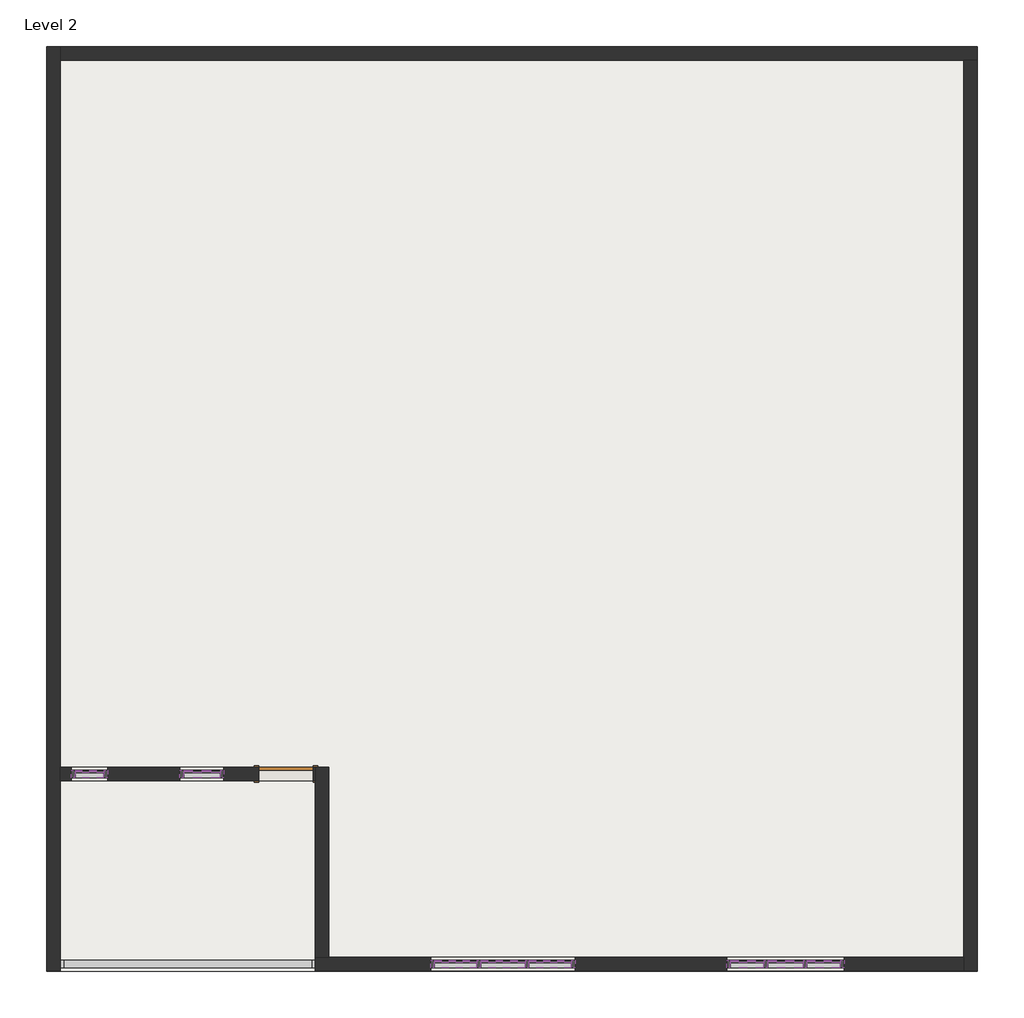
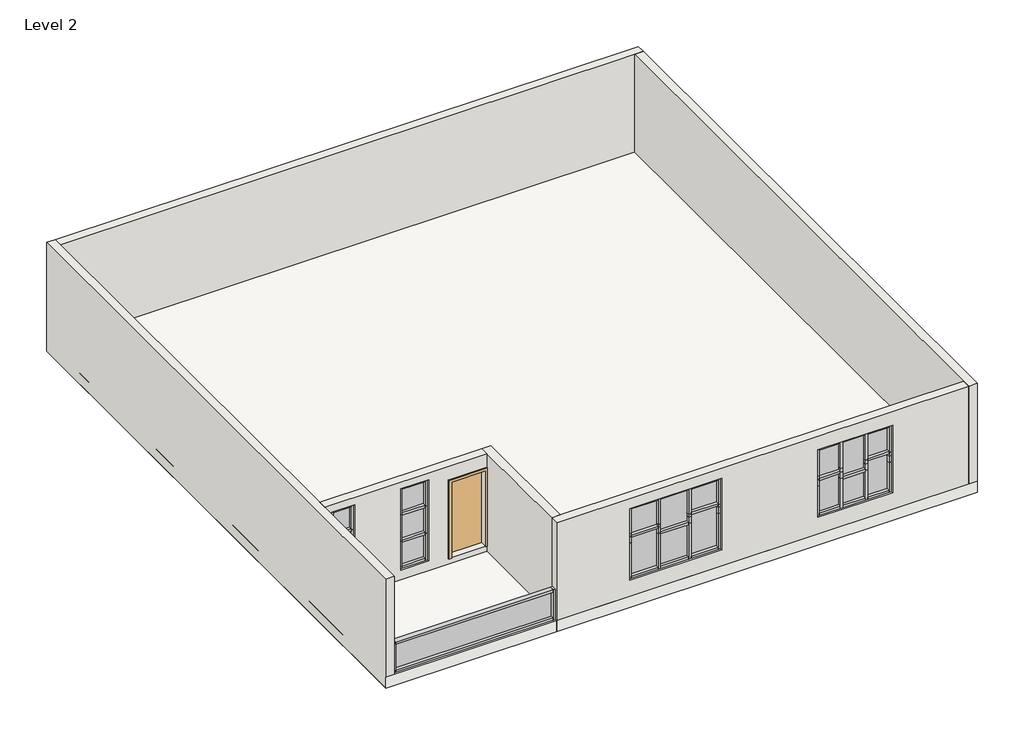
# One storey: 74 members, 19 plates, 6 walls, 1 door, 1 roof.
"""IFC4 building model written with IfcOpenShell, lengths in millimetres."""

from ifc_helpers import new_model, si_unit, frame, origin, place, context, project, spatial, polyline, outline, extrude, faceted_brep, transform, mapped, element, save
from components import door_0ca8825f, member_3d7cb871, member_6103f85b, member_00d00b53, member_86293703, member_cfc5edb3, member_a400357f, member_6f432376, member_abeaf8ac, member_798d6cad, member_9d02be77, member_7007ad49, member_86d06fe4, member_323df77c, member_fb13da3b, member_d92184fb, member_86adc6a2, member_2118ea0c, member_92f44db0, member_44fc35f8, member_a1032ffb, member_2251cb41, member_9a1a11af, member_7982986b, member_74f949a7, member_09784a4a, member_ee585a1e, member_f8dc38bf, member_3f0e0172, member_39ae6cfa, member_86c371d5, system_panel_glazed_a2969b70, system_panel_glazed_06a12247, system_panel_glazed_4710a741, system_panel_glazed_6f1997f1, system_panel_glazed_71cd45ac, system_panel_glazed_e7b2ff25, system_panel_glazed_4fbea3b4, system_panel_glazed_12683933, system_panel_glazed_3f655f72, system_panel_glazed_72d2109d, system_panel_glazed_9ec27a3c, system_panel_glazed_53cab8c3, system_panel_glazed_a0fb9759, system_panel_glazed_76104635, system_panel_glazed_cd499e62, system_panel_glazed_4a2f6317, system_panel_glazed_4f9242a6

model = new_model("IFC4")

# Units and contexts
model_context = context("Model", 3, world=origin())
ifc_project = project(units=[si_unit("LENGTHUNIT", "METRE", prefix="MILLI")], contexts=[model_context])

# Site, building, storey
site = spatial("IfcSite", under=ifc_project)
building = spatial("IfcBuilding", under=site)
storey = spatial("IfcBuildingStorey", under=building, Name="Level 2", Elevation=3048.0)

# Door
placement = place(None, origin())
door_shape = door_0ca8825f(model_context)
element("IfcDoor", 1, ObjectType="Single-Flush : 36\" x 84\"", at=placement, inside=storey, context=model_context, shape_type="MappedRepresentation", body=[
    mapped(door_shape, transform((-15283.714323, -10539.4538163, 3505.2), x_axis=(1.0, 0.0, 0.0), y_axis=(0.0, 1.0, 0.0), z_axis=(0.0, 0.0, 1.0))),
])

# Members
member_shape = member_3d7cb871(model_context)
element("IfcMember", 2, ObjectType="Rectangular Mullion : 2.5\" x 5\" rectangular", at=placement, inside=storey, context=model_context, shape_type="MappedRepresentation", body=[
    mapped(member_shape, transform((-12845.314323, -13739.8538163, 5060.9680142), x_axis=(-1.0, 0.0, 0.0), y_axis=(0.0, -1.0, 0.0), z_axis=(0.0, 0.0, 1.0))),
])
member_2_shape = member_6103f85b(model_context)
element("IfcMember", 3, ObjectType="Rectangular Mullion : 2.5\" x 5\" rectangular", at=placement, inside=storey, context=model_context, shape_type="MappedRepresentation", body=[
    mapped(member_2_shape, transform((-7225.564323, -13739.8538163, 4831.3724927), x_axis=(0.0, 0.0, 1.0), y_axis=(0.0, -1.0, 0.0), z_axis=(1.0, 0.0, 0.0))),
])
element("IfcMember", 4, ObjectType="Rectangular Mullion : 2.5\" x 5\" rectangular", at=placement, inside=storey, context=model_context, shape_type="MappedRepresentation", body=[
    mapped(member_2_shape, transform((-5936.514323, -13739.8538163, 4932.9724927), x_axis=(0.0, 0.0, 1.0), y_axis=(0.0, -1.0, 0.0), z_axis=(1.0, 0.0, 0.0))),
])
member_3_shape = member_00d00b53(model_context)
element("IfcMember", 5, ObjectType="Rectangular Mullion : 2.5\" x 5\" rectangular", at=placement, inside=storey, context=model_context, shape_type="MappedRepresentation", body=[
    mapped(member_3_shape, transform((-12032.514323, -13739.8538163, 4984.7680142), x_axis=(1.0, 0.0, 0.0), y_axis=(0.0, -1.0, 0.0), z_axis=(0.0, 0.0, -1.0))),
])
member_4_shape = member_86293703(model_context)
element("IfcMember", 6, ObjectType="Rectangular Mullion : 2.5\" x 5\" rectangular", at=placement, inside=storey, context=model_context, shape_type="MappedRepresentation", body=[
    mapped(member_4_shape, transform((-6565.164323, -13739.8538163, 4653.5724927), x_axis=(0.0, 0.0, 1.0), y_axis=(0.0, -1.0, 0.0), z_axis=(1.0, 0.0, 0.0))),
])
member_5_shape = member_cfc5edb3(model_context)
element("IfcMember", 7, ObjectType="Rectangular Mullion : 2.5\" x 5\" rectangular", at=placement, inside=storey, context=model_context, shape_type="MappedRepresentation", body=[
    mapped(member_5_shape, transform((-7193.814323, -13739.8538163, 4831.3724927), x_axis=(1.0, 0.0, 0.0), y_axis=(0.0, -1.0, 0.0), z_axis=(0.0, 0.0, -1.0))),
])
element("IfcMember", 8, ObjectType="Rectangular Mullion : 2.5\" x 5\" rectangular", at=placement, inside=storey, context=model_context, shape_type="MappedRepresentation", body=[
    mapped(member_3_shape, transform((-11219.714323, -13739.8538163, 4984.7680142), x_axis=(1.0, 0.0, 0.0), y_axis=(0.0, -1.0, 0.0), z_axis=(0.0, 0.0, -1.0))),
])
member_6_shape = member_a400357f(model_context)
element("IfcMember", 9, ObjectType="Rectangular Mullion : 2.5\" x 5\" rectangular", at=placement, inside=storey, context=model_context, shape_type="MappedRepresentation", body=[
    mapped(member_6_shape, transform((-7162.064323, -13739.8538163, 3815.3724927), x_axis=(0.0, 0.0, -1.0), y_axis=(0.0, -1.0, 0.0), z_axis=(-1.0, 0.0, 0.0))),
])
member_7_shape = member_6f432376(model_context)
element("IfcMember", 10, ObjectType="Rectangular Mullion : 2.5\" x 5\" rectangular", at=placement, inside=storey, context=model_context, shape_type="MappedRepresentation", body=[
    mapped(member_7_shape, transform((-6501.664323, -13739.8538163, 3815.3724927), x_axis=(0.0, 0.0, -1.0), y_axis=(0.0, -1.0, 0.0), z_axis=(-1.0, 0.0, 0.0))),
])
element("IfcMember", 11, ObjectType="Rectangular Mullion : 2.5\" x 5\" rectangular", at=placement, inside=storey, context=model_context, shape_type="MappedRepresentation", body=[
    mapped(member_7_shape, transform((-7790.714323, -13739.8538163, 3815.3724927), x_axis=(0.0, 0.0, -1.0), y_axis=(0.0, -1.0, 0.0), z_axis=(-1.0, 0.0, 0.0))),
])
element("IfcMember", 12, ObjectType="Rectangular Mullion : 2.5\" x 5\" rectangular", at=placement, inside=storey, context=model_context, shape_type="MappedRepresentation", body=[
    mapped(member_7_shape, transform((-7225.564323, -13739.8538163, 5713.2534541), x_axis=(0.0, 0.0, 1.0), y_axis=(0.0, -1.0, 0.0), z_axis=(1.0, 0.0, 0.0))),
])
element("IfcMember", 13, ObjectType="Rectangular Mullion : 2.5\" x 5\" rectangular", at=placement, inside=storey, context=model_context, shape_type="MappedRepresentation", body=[
    mapped(member_7_shape, transform((-5936.514323, -13739.8538163, 5713.2534541), x_axis=(0.0, 0.0, 1.0), y_axis=(0.0, -1.0, 0.0), z_axis=(1.0, 0.0, 0.0))),
])
element("IfcMember", 14, ObjectType="Rectangular Mullion : 2.5\" x 5\" rectangular", at=placement, inside=storey, context=model_context, shape_type="MappedRepresentation", body=[
    mapped(member_6_shape, transform((-6565.164323, -13739.8538163, 5713.2534541), x_axis=(0.0, 0.0, 1.0), y_axis=(0.0, -1.0, 0.0), z_axis=(1.0, 0.0, 0.0))),
])
member_8_shape = member_abeaf8ac(model_context)
element("IfcMember", 15, ObjectType="Rectangular Mullion : 2.5\" x 5\" rectangular", at=placement, inside=storey, context=model_context, shape_type="MappedRepresentation", body=[
    mapped(member_8_shape, transform((-12064.264323, -13739.8538163, 4984.7680142), x_axis=(0.0, 0.0, 1.0), y_axis=(0.0, -1.0, 0.0), z_axis=(1.0, 0.0, 0.0))),
])
element("IfcMember", 16, ObjectType="Rectangular Mullion : 2.5\" x 5\" rectangular", at=placement, inside=storey, context=model_context, shape_type="MappedRepresentation", body=[
    mapped(member_8_shape, transform((-10470.414323, -13739.8538163, 5060.9680142), x_axis=(0.0, 0.0, 1.0), y_axis=(0.0, -1.0, 0.0), z_axis=(1.0, 0.0, 0.0))),
])
member_9_shape = member_798d6cad(model_context)
element("IfcMember", 17, ObjectType="Rectangular Mullion : 2.5\" x 5\" rectangular", at=placement, inside=storey, context=model_context, shape_type="MappedRepresentation", body=[
    mapped(member_9_shape, transform((-11251.464323, -13739.8538163, 4806.9680142), x_axis=(0.0, 0.0, 1.0), y_axis=(0.0, -1.0, 0.0), z_axis=(1.0, 0.0, 0.0))),
])
member_10_shape = member_9d02be77(model_context)
element("IfcMember", 18, ObjectType="Rectangular Mullion : 2.5\" x 5\" rectangular", at=placement, inside=storey, context=model_context, shape_type="MappedRepresentation", body=[
    mapped(member_10_shape, transform((-12000.764323, -13739.8538163, 3802.3510982), x_axis=(0.0, 0.0, -1.0), y_axis=(0.0, -1.0, 0.0), z_axis=(-1.0, 0.0, 0.0))),
])
member_11_shape = member_7007ad49(model_context)
element("IfcMember", 19, ObjectType="Rectangular Mullion : 2.5\" x 5\" rectangular", at=placement, inside=storey, context=model_context, shape_type="MappedRepresentation", body=[
    mapped(member_11_shape, transform((-11187.964323, -13739.8538163, 3802.3510982), x_axis=(0.0, 0.0, -1.0), y_axis=(0.0, -1.0, 0.0), z_axis=(-1.0, 0.0, 0.0))),
])
element("IfcMember", 20, ObjectType="Rectangular Mullion : 2.5\" x 5\" rectangular", at=placement, inside=storey, context=model_context, shape_type="MappedRepresentation", body=[
    mapped(member_11_shape, transform((-12781.814323, -13739.8538163, 3802.3510982), x_axis=(0.0, 0.0, -1.0), y_axis=(0.0, -1.0, 0.0), z_axis=(-1.0, 0.0, 0.0))),
])
element("IfcMember", 21, ObjectType="Rectangular Mullion : 2.5\" x 5\" rectangular", at=placement, inside=storey, context=model_context, shape_type="MappedRepresentation", body=[
    mapped(member_shape, transform((-10406.914323, -13739.8538163, 4984.7680142), x_axis=(1.0, 0.0, 0.0), y_axis=(0.0, -1.0, 0.0), z_axis=(0.0, 0.0, -1.0))),
])
element("IfcMember", 22, ObjectType="Rectangular Mullion : 2.5\" x 5\" rectangular", at=placement, inside=storey, context=model_context, shape_type="MappedRepresentation", body=[
    mapped(member_10_shape, transform((-11251.464323, -13739.8538163, 5811.5849303), x_axis=(0.0, 0.0, 1.0), y_axis=(0.0, -1.0, 0.0), z_axis=(1.0, 0.0, 0.0))),
])
element("IfcMember", 23, ObjectType="Rectangular Mullion : 2.5\" x 5\" rectangular", at=placement, inside=storey, context=model_context, shape_type="MappedRepresentation", body=[
    mapped(member_11_shape, transform((-12064.264323, -13739.8538163, 5811.5849303), x_axis=(0.0, 0.0, 1.0), y_axis=(0.0, -1.0, 0.0), z_axis=(1.0, 0.0, 0.0))),
])
element("IfcMember", 24, ObjectType="Rectangular Mullion : 2.5\" x 5\" rectangular", at=placement, inside=storey, context=model_context, shape_type="MappedRepresentation", body=[
    mapped(member_11_shape, transform((-10470.414323, -13739.8538163, 5811.5849303), x_axis=(0.0, 0.0, 1.0), y_axis=(0.0, -1.0, 0.0), z_axis=(1.0, 0.0, 0.0))),
])
member_12_shape = member_86d06fe4(model_context)
element("IfcMember", 25, ObjectType="Rectangular Mullion : 2.5\" x 5\" rectangular", at=placement, inside=storey, context=model_context, shape_type="MappedRepresentation", body=[
    mapped(member_12_shape, transform((-18357.114323, -10539.4538163, 5888.5899521), x_axis=(0.0, 0.0, 1.0), y_axis=(0.0, -1.0, 0.0), z_axis=(1.0, 0.0, 0.0))),
])
member_13_shape = member_323df77c(model_context)
element("IfcMember", 26, ObjectType="Rectangular Mullion : 2.5\" x 5\" rectangular", at=placement, inside=storey, context=model_context, shape_type="MappedRepresentation", body=[
    mapped(member_13_shape, transform((-18357.114323, -10539.4538163, 5168.781413), x_axis=(0.0, 0.0, 1.0), y_axis=(0.0, -1.0, 0.0), z_axis=(1.0, 0.0, 0.0))),
])
element("IfcMember", 27, ObjectType="Rectangular Mullion : 2.5\" x 5\" rectangular", at=placement, inside=storey, context=model_context, shape_type="MappedRepresentation", body=[
    mapped(member_13_shape, transform((-18357.114323, -10539.4538163, 4448.9728739), x_axis=(0.0, 0.0, 1.0), y_axis=(0.0, -1.0, 0.0), z_axis=(1.0, 0.0, 0.0))),
])
element("IfcMember", 28, ObjectType="Rectangular Mullion : 2.5\" x 5\" rectangular", at=placement, inside=storey, context=model_context, shape_type="MappedRepresentation", body=[
    mapped(member_12_shape, transform((-18839.714323, -10539.4538163, 3729.1643349), x_axis=(0.0, 0.0, -1.0), y_axis=(0.0, -1.0, 0.0), z_axis=(-1.0, 0.0, 0.0))),
])
member_14_shape = member_fb13da3b(model_context)
element("IfcMember", 29, ObjectType="Rectangular Mullion : 2.5\" x 5\" rectangular", at=placement, inside=storey, context=model_context, shape_type="MappedRepresentation", body=[
    mapped(member_14_shape, transform((-7854.214323, -13739.8538163, 4932.9724927), x_axis=(-1.0, 0.0, 0.0), y_axis=(0.0, -1.0, 0.0), z_axis=(0.0, 0.0, 1.0))),
])
member_15_shape = member_d92184fb(model_context)
element("IfcMember", 30, ObjectType="Rectangular Mullion : 2.5\" x 5\" rectangular", at=placement, inside=storey, context=model_context, shape_type="MappedRepresentation", body=[
    mapped(member_15_shape, transform((-7854.214323, -13739.8538163, 4831.3724927), x_axis=(-1.0, 0.0, 0.0), y_axis=(0.0, -1.0, 0.0), z_axis=(0.0, 0.0, 1.0))),
])
element("IfcMember", 31, ObjectType="Rectangular Mullion : 2.5\" x 5\" rectangular", at=placement, inside=storey, context=model_context, shape_type="MappedRepresentation", body=[
    mapped(member_15_shape, transform((-12845.314323, -13739.8538163, 4984.7680142), x_axis=(-1.0, 0.0, 0.0), y_axis=(0.0, -1.0, 0.0), z_axis=(0.0, 0.0, 1.0))),
])
member_16_shape = member_86adc6a2(model_context)
element("IfcMember", 32, ObjectType="Rectangular Mullion : 2.5\" x 5\" rectangular", at=placement, inside=storey, context=model_context, shape_type="MappedRepresentation", body=[
    mapped(member_16_shape, transform((-7854.214323, -13739.8538163, 4653.5724927), x_axis=(-1.0, 0.0, 0.0), y_axis=(0.0, -1.0, 0.0), z_axis=(0.0, 0.0, 1.0))),
])
member_17_shape = member_2118ea0c(model_context)
element("IfcMember", 33, ObjectType="Rectangular Mullion : 2.5\" x 5\" rectangular", at=placement, inside=storey, context=model_context, shape_type="MappedRepresentation", body=[
    mapped(member_17_shape, transform((-7193.814323, -13739.8538163, 4653.5724927), x_axis=(1.0, 0.0, 0.0), y_axis=(0.0, -1.0, 0.0), z_axis=(0.0, 0.0, -1.0))),
])
element("IfcMember", 34, ObjectType="Rectangular Mullion : 2.5\" x 5\" rectangular", at=placement, inside=storey, context=model_context, shape_type="MappedRepresentation", body=[
    mapped(member_17_shape, transform((-12032.514323, -13739.8538163, 4806.9680142), x_axis=(1.0, 0.0, 0.0), y_axis=(0.0, -1.0, 0.0), z_axis=(0.0, 0.0, -1.0))),
])
member_18_shape = member_92f44db0(model_context)
element("IfcMember", 35, ObjectType="Rectangular Mullion : 2.5\" x 5\" rectangular", at=placement, inside=storey, context=model_context, shape_type="MappedRepresentation", body=[
    mapped(member_18_shape, transform((-7193.814323, -13739.8538163, 3815.3724927), x_axis=(1.0, 0.0, 0.0), y_axis=(0.0, -1.0, 0.0), z_axis=(0.0, 0.0, -1.0))),
])
element("IfcMember", 36, ObjectType="Rectangular Mullion : 2.5\" x 5\" rectangular", at=placement, inside=storey, context=model_context, shape_type="MappedRepresentation", body=[
    mapped(member_18_shape, transform((-6533.414323, -13739.8538163, 3815.3724927), x_axis=(1.0, 0.0, 0.0), y_axis=(0.0, -1.0, 0.0), z_axis=(0.0, 0.0, -1.0))),
])
element("IfcMember", 37, ObjectType="Rectangular Mullion : 2.5\" x 5\" rectangular", at=placement, inside=storey, context=model_context, shape_type="MappedRepresentation", body=[
    mapped(member_17_shape, transform((-6533.414323, -13739.8538163, 4653.5724927), x_axis=(1.0, 0.0, 0.0), y_axis=(0.0, -1.0, 0.0), z_axis=(0.0, 0.0, -1.0))),
])
element("IfcMember", 38, ObjectType="Rectangular Mullion : 2.5\" x 5\" rectangular", at=placement, inside=storey, context=model_context, shape_type="MappedRepresentation", body=[
    mapped(member_17_shape, transform((-11219.714323, -13739.8538163, 4806.9680142), x_axis=(1.0, 0.0, 0.0), y_axis=(0.0, -1.0, 0.0), z_axis=(0.0, 0.0, -1.0))),
])
element("IfcMember", 39, ObjectType="Rectangular Mullion : 2.5\" x 5\" rectangular", at=placement, inside=storey, context=model_context, shape_type="MappedRepresentation", body=[
    mapped(member_5_shape, transform((-6533.414323, -13739.8538163, 4831.3724927), x_axis=(1.0, 0.0, 0.0), y_axis=(0.0, -1.0, 0.0), z_axis=(0.0, 0.0, -1.0))),
])
element("IfcMember", 40, ObjectType="Rectangular Mullion : 2.5\" x 5\" rectangular", at=placement, inside=storey, context=model_context, shape_type="MappedRepresentation", body=[
    mapped(member_14_shape, transform((-5873.014323, -13739.8538163, 4831.3724927), x_axis=(1.0, 0.0, 0.0), y_axis=(0.0, -1.0, 0.0), z_axis=(0.0, 0.0, -1.0))),
])
element("IfcMember", 41, ObjectType="Rectangular Mullion : 2.5\" x 5\" rectangular", at=placement, inside=storey, context=model_context, shape_type="MappedRepresentation", body=[
    mapped(member_15_shape, transform((-5873.014323, -13739.8538163, 4653.5724927), x_axis=(1.0, 0.0, 0.0), y_axis=(0.0, -1.0, 0.0), z_axis=(0.0, 0.0, -1.0))),
])
element("IfcMember", 42, ObjectType="Rectangular Mullion : 2.5\" x 5\" rectangular", at=placement, inside=storey, context=model_context, shape_type="MappedRepresentation", body=[
    mapped(member_15_shape, transform((-10406.914323, -13739.8538163, 4806.9680142), x_axis=(1.0, 0.0, 0.0), y_axis=(0.0, -1.0, 0.0), z_axis=(0.0, 0.0, -1.0))),
])
element("IfcMember", 43, ObjectType="Rectangular Mullion : 2.5\" x 5\" rectangular", at=placement, inside=storey, context=model_context, shape_type="MappedRepresentation", body=[
    mapped(member_16_shape, transform((-5873.014323, -13739.8538163, 3815.3724927), x_axis=(1.0, 0.0, 0.0), y_axis=(0.0, -1.0, 0.0), z_axis=(0.0, 0.0, -1.0))),
])
member_19_shape = member_44fc35f8(model_context)
element("IfcMember", 44, ObjectType="Rectangular Mullion : 2.5\" x 5\" rectangular", at=placement, inside=storey, context=model_context, shape_type="MappedRepresentation", body=[
    mapped(member_19_shape, transform((-7193.814323, -13739.8538163, 4932.9724927), x_axis=(1.0, 0.0, 0.0), y_axis=(0.0, -1.0, 0.0), z_axis=(0.0, 0.0, -1.0))),
])
element("IfcMember", 45, ObjectType="Rectangular Mullion : 2.5\" x 5\" rectangular", at=placement, inside=storey, context=model_context, shape_type="MappedRepresentation", body=[
    mapped(member_19_shape, transform((-6533.414323, -13739.8538163, 4932.9724927), x_axis=(1.0, 0.0, 0.0), y_axis=(0.0, -1.0, 0.0), z_axis=(0.0, 0.0, -1.0))),
])
member_20_shape = member_a1032ffb(model_context)
element("IfcMember", 46, ObjectType="Rectangular Mullion : 2.5\" x 5\" rectangular", at=placement, inside=storey, context=model_context, shape_type="MappedRepresentation", body=[
    mapped(member_20_shape, transform((-7854.214323, -13739.8538163, 5713.2534541), x_axis=(-1.0, 0.0, 0.0), y_axis=(0.0, -1.0, 0.0), z_axis=(0.0, 0.0, 1.0))),
])
element("IfcMember", 47, ObjectType="Rectangular Mullion : 2.5\" x 5\" rectangular", at=placement, inside=storey, context=model_context, shape_type="MappedRepresentation", body=[
    mapped(member_20_shape, transform((-5873.014323, -13739.8538163, 4932.9724927), x_axis=(1.0, 0.0, 0.0), y_axis=(0.0, -1.0, 0.0), z_axis=(0.0, 0.0, -1.0))),
])
member_21_shape = member_2251cb41(model_context)
element("IfcMember", 48, ObjectType="Rectangular Mullion : 2.5\" x 5\" rectangular", at=placement, inside=storey, context=model_context, shape_type="MappedRepresentation", body=[
    mapped(member_21_shape, transform((-12032.514323, -13739.8538163, 3802.3510982), x_axis=(1.0, 0.0, 0.0), y_axis=(0.0, -1.0, 0.0), z_axis=(0.0, 0.0, -1.0))),
])
element("IfcMember", 49, ObjectType="Rectangular Mullion : 2.5\" x 5\" rectangular", at=placement, inside=storey, context=model_context, shape_type="MappedRepresentation", body=[
    mapped(member_21_shape, transform((-11219.714323, -13739.8538163, 3802.3510982), x_axis=(1.0, 0.0, 0.0), y_axis=(0.0, -1.0, 0.0), z_axis=(0.0, 0.0, -1.0))),
])
member_22_shape = member_9a1a11af(model_context)
element("IfcMember", 50, ObjectType="Rectangular Mullion : 2.5\" x 5\" rectangular", at=placement, inside=storey, context=model_context, shape_type="MappedRepresentation", body=[
    mapped(member_22_shape, transform((-12845.314323, -13739.8538163, 4806.9680142), x_axis=(-1.0, 0.0, 0.0), y_axis=(0.0, -1.0, 0.0), z_axis=(0.0, 0.0, 1.0))),
])
member_23_shape = member_7982986b(model_context)
element("IfcMember", 51, ObjectType="Rectangular Mullion : 2.5\" x 5\" rectangular", at=placement, inside=storey, context=model_context, shape_type="MappedRepresentation", body=[
    mapped(member_23_shape, transform((-12032.514323, -13739.8538163, 5060.9680142), x_axis=(1.0, 0.0, 0.0), y_axis=(0.0, -1.0, 0.0), z_axis=(0.0, 0.0, -1.0))),
])
element("IfcMember", 52, ObjectType="Rectangular Mullion : 2.5\" x 5\" rectangular", at=placement, inside=storey, context=model_context, shape_type="MappedRepresentation", body=[
    mapped(member_23_shape, transform((-11219.714323, -13739.8538163, 5060.9680142), x_axis=(1.0, 0.0, 0.0), y_axis=(0.0, -1.0, 0.0), z_axis=(0.0, 0.0, -1.0))),
])
member_24_shape = member_74f949a7(model_context)
element("IfcMember", 53, ObjectType="Rectangular Mullion : 2.5\" x 5\" rectangular", at=placement, inside=storey, context=model_context, shape_type="MappedRepresentation", body=[
    mapped(member_24_shape, transform((-12845.314323, -13739.8538163, 5811.5849303), x_axis=(-1.0, 0.0, 0.0), y_axis=(0.0, -1.0, 0.0), z_axis=(0.0, 0.0, 1.0))),
])
element("IfcMember", 54, ObjectType="Rectangular Mullion : 2.5\" x 5\" rectangular", at=placement, inside=storey, context=model_context, shape_type="MappedRepresentation", body=[
    mapped(member_24_shape, transform((-10406.914323, -13739.8538163, 5060.9680142), x_axis=(1.0, 0.0, 0.0), y_axis=(0.0, -1.0, 0.0), z_axis=(0.0, 0.0, -1.0))),
])
element("IfcMember", 55, ObjectType="Rectangular Mullion : 2.5\" x 5\" rectangular", at=placement, inside=storey, context=model_context, shape_type="MappedRepresentation", body=[
    mapped(member_22_shape, transform((-10406.914323, -13739.8538163, 3802.3510982), x_axis=(1.0, 0.0, 0.0), y_axis=(0.0, -1.0, 0.0), z_axis=(0.0, 0.0, -1.0))),
])
member_25_shape = member_09784a4a(model_context)
element("IfcMember", 56, ObjectType="Rectangular Mullion : 2.5\" x 5\" rectangular", at=placement, inside=storey, context=model_context, shape_type="MappedRepresentation", body=[
    mapped(member_25_shape, transform((-18903.214323, -10539.4538163, 5168.781413), x_axis=(-1.0, 0.0, 0.0), y_axis=(0.0, -1.0, 0.0), z_axis=(0.0, 0.0, 1.0))),
])
element("IfcMember", 57, ObjectType="Rectangular Mullion : 2.5\" x 5\" rectangular", at=placement, inside=storey, context=model_context, shape_type="MappedRepresentation", body=[
    mapped(member_25_shape, transform((-18903.214323, -10539.4538163, 4448.9728739), x_axis=(-1.0, 0.0, 0.0), y_axis=(0.0, -1.0, 0.0), z_axis=(0.0, 0.0, 1.0))),
])
element("IfcMember", 58, ObjectType="Rectangular Mullion : 2.5\" x 5\" rectangular", at=placement, inside=storey, context=model_context, shape_type="MappedRepresentation", body=[
    mapped(member_25_shape, transform((-18903.214323, -10539.4538163, 5888.5899521), x_axis=(-1.0, 0.0, 0.0), y_axis=(0.0, -1.0, 0.0), z_axis=(0.0, 0.0, 1.0))),
])
element("IfcMember", 59, ObjectType="Rectangular Mullion : 2.5\" x 5\" rectangular", at=placement, inside=storey, context=model_context, shape_type="MappedRepresentation", body=[
    mapped(member_25_shape, transform((-18293.614323, -10539.4538163, 4448.9728739), x_axis=(1.0, 0.0, 0.0), y_axis=(0.0, -1.0, 0.0), z_axis=(0.0, 0.0, -1.0))),
])
element("IfcMember", 60, ObjectType="Rectangular Mullion : 2.5\" x 5\" rectangular", at=placement, inside=storey, context=model_context, shape_type="MappedRepresentation", body=[
    mapped(member_25_shape, transform((-18293.614323, -10539.4538163, 5168.781413), x_axis=(1.0, 0.0, 0.0), y_axis=(0.0, -1.0, 0.0), z_axis=(0.0, 0.0, -1.0))),
])
element("IfcMember", 61, ObjectType="Rectangular Mullion : 2.5\" x 5\" rectangular", at=placement, inside=storey, context=model_context, shape_type="MappedRepresentation", body=[
    mapped(member_25_shape, transform((-18293.614323, -10539.4538163, 3729.1643349), x_axis=(1.0, 0.0, 0.0), y_axis=(0.0, -1.0, 0.0), z_axis=(0.0, 0.0, -1.0))),
])
member_26_shape = member_ee585a1e(model_context)
element("IfcMember", 62, ObjectType="Rectangular Mullion : 2.5\" x 5\" rectangular", at=placement, inside=storey, context=model_context, shape_type="MappedRepresentation", body=[
    mapped(member_26_shape, transform((-17074.414323, -10539.4538163, 5906.3837859), x_axis=(-1.0, 0.0, 0.0), y_axis=(0.0, -1.0, 0.0), z_axis=(0.0, 0.0, 1.0))),
])
member_27_shape = member_f8dc38bf(model_context)
element("IfcMember", 63, ObjectType="Rectangular Mullion : 2.5\" x 5\" rectangular", at=placement, inside=storey, context=model_context, shape_type="MappedRepresentation", body=[
    mapped(member_27_shape, transform((-16394.964323, -10539.4538163, 5145.5335319), x_axis=(0.0, 0.0, 1.0), y_axis=(0.0, -1.0, 0.0), z_axis=(1.0, 0.0, 0.0))),
])
element("IfcMember", 64, ObjectType="Rectangular Mullion : 2.5\" x 5\" rectangular", at=placement, inside=storey, context=model_context, shape_type="MappedRepresentation", body=[
    mapped(member_27_shape, transform((-16394.964323, -10539.4538163, 4384.6832779), x_axis=(0.0, 0.0, 1.0), y_axis=(0.0, -1.0, 0.0), z_axis=(1.0, 0.0, 0.0))),
])
member_28_shape = member_3f0e0172(model_context)
element("IfcMember", 65, ObjectType="Rectangular Mullion : 2.5\" x 5\" rectangular", at=placement, inside=storey, context=model_context, shape_type="MappedRepresentation", body=[
    mapped(member_28_shape, transform((-16394.964323, -10539.4538163, 5906.3837859), x_axis=(0.0, 0.0, 1.0), y_axis=(0.0, -1.0, 0.0), z_axis=(1.0, 0.0, 0.0))),
])
element("IfcMember", 66, ObjectType="Rectangular Mullion : 2.5\" x 5\" rectangular", at=placement, inside=storey, context=model_context, shape_type="MappedRepresentation", body=[
    mapped(member_26_shape, transform((-16331.464323, -10539.4538163, 5145.5335319), x_axis=(1.0, 0.0, 0.0), y_axis=(0.0, -1.0, 0.0), z_axis=(0.0, 0.0, -1.0))),
])
element("IfcMember", 67, ObjectType="Rectangular Mullion : 2.5\" x 5\" rectangular", at=placement, inside=storey, context=model_context, shape_type="MappedRepresentation", body=[
    mapped(member_26_shape, transform((-17074.414323, -10539.4538163, 5145.5335319), x_axis=(-1.0, 0.0, 0.0), y_axis=(0.0, -1.0, 0.0), z_axis=(0.0, 0.0, 1.0))),
])
element("IfcMember", 68, ObjectType="Rectangular Mullion : 2.5\" x 5\" rectangular", at=placement, inside=storey, context=model_context, shape_type="MappedRepresentation", body=[
    mapped(member_26_shape, transform((-16331.464323, -10539.4538163, 4384.6832779), x_axis=(1.0, 0.0, 0.0), y_axis=(0.0, -1.0, 0.0), z_axis=(0.0, 0.0, -1.0))),
])
element("IfcMember", 69, ObjectType="Rectangular Mullion : 2.5\" x 5\" rectangular", at=placement, inside=storey, context=model_context, shape_type="MappedRepresentation", body=[
    mapped(member_28_shape, transform((-17010.914323, -10539.4538163, 3623.8330239), x_axis=(0.0, 0.0, -1.0), y_axis=(0.0, -1.0, 0.0), z_axis=(-1.0, 0.0, 0.0))),
])
element("IfcMember", 70, ObjectType="Rectangular Mullion : 2.5\" x 5\" rectangular", at=placement, inside=storey, context=model_context, shape_type="MappedRepresentation", body=[
    mapped(member_26_shape, transform((-17074.414323, -10539.4538163, 4384.6832779), x_axis=(-1.0, 0.0, 0.0), y_axis=(0.0, -1.0, 0.0), z_axis=(0.0, 0.0, 1.0))),
])
element("IfcMember", 71, ObjectType="Rectangular Mullion : 2.5\" x 5\" rectangular", at=placement, inside=storey, context=model_context, shape_type="MappedRepresentation", body=[
    mapped(member_26_shape, transform((-16331.464323, -10539.4538163, 3623.8330239), x_axis=(1.0, 0.0, 0.0), y_axis=(0.0, -1.0, 0.0), z_axis=(0.0, 0.0, -1.0))),
])
member_29_shape = member_39ae6cfa(model_context)
element("IfcMember", 72, ObjectType="Rectangular Mullion : 2.5\" x 5\" rectangular", at=placement, inside=storey, context=model_context, shape_type="MappedRepresentation", body=[
    mapped(member_29_shape, transform((-19093.714323, -13739.8538163, 4204.113055), x_axis=(-1.0, 0.0, 0.0), y_axis=(0.0, -1.0, 0.0), z_axis=(0.0, 0.0, 1.0))),
])
member_30_shape = member_86c371d5(model_context)
element("IfcMember", 73, ObjectType="Rectangular Mullion : 2.5\" x 5\" rectangular", at=placement, inside=storey, context=model_context, shape_type="MappedRepresentation", body=[
    mapped(member_30_shape, transform((-14851.914323, -13739.8538163, 4204.113055), x_axis=(0.0, 0.0, 1.0), y_axis=(0.0, -1.0, 0.0), z_axis=(1.0, 0.0, 0.0))),
])
element("IfcMember", 74, ObjectType="Rectangular Mullion : 2.5\" x 5\" rectangular", at=placement, inside=storey, context=model_context, shape_type="MappedRepresentation", body=[
    mapped(member_30_shape, transform((-19030.214323, -13739.8538163, 3352.8), x_axis=(0.0, 0.0, -1.0), y_axis=(0.0, -1.0, 0.0), z_axis=(-1.0, 0.0, 0.0))),
])
element("IfcMember", 75, ObjectType="Rectangular Mullion : 2.5\" x 5\" rectangular", at=placement, inside=storey, context=model_context, shape_type="MappedRepresentation", body=[
    mapped(member_29_shape, transform((-14788.414323, -13739.8538163, 3352.8), x_axis=(1.0, 0.0, 0.0), y_axis=(0.0, -1.0, 0.0), z_axis=(0.0, 0.0, -1.0))),
])

# Plates
system_panel_glazed_shape = system_panel_glazed_a2969b70(model_context)
element("IfcPlate", 76, ObjectType="System Panel : Glazed", at=placement, inside=storey, context=model_context, shape_type="MappedRepresentation", body=[
    mapped(system_panel_glazed_shape, transform((-7508.139323, -13739.8538163, 3878.8724927), x_axis=(1.0, 0.0, 0.0), y_axis=(0.0, 1.0, 0.0), z_axis=(0.0, 0.0, 1.0))),
])
system_panel_glazed_2_shape = system_panel_glazed_06a12247(model_context)
element("IfcPlate", 77, ObjectType="System Panel : Glazed", at=placement, inside=storey, context=model_context, shape_type="MappedRepresentation", body=[
    mapped(system_panel_glazed_2_shape, transform((-6863.614323, -13739.8538163, 3878.8724927), x_axis=(1.0, 0.0, 0.0), y_axis=(0.0, 1.0, 0.0), z_axis=(0.0, 0.0, 1.0))),
])
system_panel_glazed_3_shape = system_panel_glazed_4710a741(model_context)
element("IfcPlate", 78, ObjectType="System Panel : Glazed", at=placement, inside=storey, context=model_context, shape_type="MappedRepresentation", body=[
    mapped(system_panel_glazed_3_shape, transform((-6219.089323, -13739.8538163, 3878.8724927), x_axis=(1.0, 0.0, 0.0), y_axis=(0.0, 1.0, 0.0), z_axis=(0.0, 0.0, 1.0))),
])
system_panel_glazed_4_shape = system_panel_glazed_6f1997f1(model_context)
element("IfcPlate", 79, ObjectType="System Panel : Glazed", at=placement, inside=storey, context=model_context, shape_type="MappedRepresentation", body=[
    mapped(system_panel_glazed_4_shape, transform((-6863.614323, -13739.8538163, 4685.3224927), x_axis=(1.0, 0.0, 0.0), y_axis=(0.0, 1.0, 0.0), z_axis=(0.0, 0.0, 1.0))),
])
system_panel_glazed_5_shape = system_panel_glazed_71cd45ac(model_context)
element("IfcPlate", 80, ObjectType="System Panel : Glazed", at=placement, inside=storey, context=model_context, shape_type="MappedRepresentation", body=[
    mapped(system_panel_glazed_5_shape, transform((-7508.139323, -13739.8538163, 4863.1224927), x_axis=(1.0, 0.0, 0.0), y_axis=(0.0, 1.0, 0.0), z_axis=(0.0, 0.0, 1.0))),
])
system_panel_glazed_6_shape = system_panel_glazed_e7b2ff25(model_context)
element("IfcPlate", 81, ObjectType="System Panel : Glazed", at=placement, inside=storey, context=model_context, shape_type="MappedRepresentation", body=[
    mapped(system_panel_glazed_6_shape, transform((-6219.089323, -13739.8538163, 4964.7224927), x_axis=(1.0, 0.0, 0.0), y_axis=(0.0, 1.0, 0.0), z_axis=(0.0, 0.0, 1.0))),
])
system_panel_glazed_7_shape = system_panel_glazed_4fbea3b4(model_context)
element("IfcPlate", 82, ObjectType="System Panel : Glazed", at=placement, inside=storey, context=model_context, shape_type="MappedRepresentation", body=[
    mapped(system_panel_glazed_7_shape, transform((-12423.039323, -13739.8538163, 3865.8510982), x_axis=(1.0, 0.0, 0.0), y_axis=(0.0, 1.0, 0.0), z_axis=(0.0, 0.0, 1.0))),
])
system_panel_glazed_8_shape = system_panel_glazed_12683933(model_context)
element("IfcPlate", 83, ObjectType="System Panel : Glazed", at=placement, inside=storey, context=model_context, shape_type="MappedRepresentation", body=[
    mapped(system_panel_glazed_8_shape, transform((-11626.114323, -13739.8538163, 3865.8510982), x_axis=(1.0, 0.0, 0.0), y_axis=(0.0, 1.0, 0.0), z_axis=(0.0, 0.0, 1.0))),
])
system_panel_glazed_9_shape = system_panel_glazed_3f655f72(model_context)
element("IfcPlate", 84, ObjectType="System Panel : Glazed", at=placement, inside=storey, context=model_context, shape_type="MappedRepresentation", body=[
    mapped(system_panel_glazed_9_shape, transform((-11626.114323, -13739.8538163, 4838.7180142), x_axis=(1.0, 0.0, 0.0), y_axis=(0.0, 1.0, 0.0), z_axis=(0.0, 0.0, 1.0))),
])
system_panel_glazed_10_shape = system_panel_glazed_72d2109d(model_context)
element("IfcPlate", 85, ObjectType="System Panel : Glazed", at=placement, inside=storey, context=model_context, shape_type="MappedRepresentation", body=[
    mapped(system_panel_glazed_10_shape, transform((-12423.039323, -13739.8538163, 5016.5180142), x_axis=(1.0, 0.0, 0.0), y_axis=(0.0, 1.0, 0.0), z_axis=(0.0, 0.0, 1.0))),
])
system_panel_glazed_11_shape = system_panel_glazed_9ec27a3c(model_context)
element("IfcPlate", 86, ObjectType="System Panel : Glazed", at=placement, inside=storey, context=model_context, shape_type="MappedRepresentation", body=[
    mapped(system_panel_glazed_11_shape, transform((-10829.189323, -13739.8538163, 3865.8510982), x_axis=(1.0, 0.0, 0.0), y_axis=(0.0, 1.0, 0.0), z_axis=(0.0, 0.0, 1.0))),
])
system_panel_glazed_12_shape = system_panel_glazed_53cab8c3(model_context)
element("IfcPlate", 87, ObjectType="System Panel : Glazed", at=placement, inside=storey, context=model_context, shape_type="MappedRepresentation", body=[
    mapped(system_panel_glazed_12_shape, transform((-10829.189323, -13739.8538163, 5092.7180142), x_axis=(1.0, 0.0, 0.0), y_axis=(0.0, 1.0, 0.0), z_axis=(0.0, 0.0, 1.0))),
])
system_panel_glazed_13_shape = system_panel_glazed_a0fb9759(model_context)
element("IfcPlate", 88, ObjectType="System Panel : Glazed", at=placement, inside=storey, context=model_context, shape_type="MappedRepresentation", body=[
    mapped(system_panel_glazed_13_shape, transform((-18598.414323, -10539.4538163, 3792.6643349), x_axis=(1.0, 0.0, 0.0), y_axis=(0.0, 1.0, 0.0), z_axis=(0.0, 0.0, 1.0))),
])
element("IfcPlate", 89, ObjectType="System Panel : Glazed", at=placement, inside=storey, context=model_context, shape_type="MappedRepresentation", body=[
    mapped(system_panel_glazed_13_shape, transform((-18598.414323, -10539.4538163, 5200.531413), x_axis=(1.0, 0.0, 0.0), y_axis=(0.0, 1.0, 0.0), z_axis=(0.0, 0.0, 1.0))),
])
system_panel_glazed_14_shape = system_panel_glazed_76104635(model_context)
element("IfcPlate", 90, ObjectType="System Panel : Glazed", at=placement, inside=storey, context=model_context, shape_type="MappedRepresentation", body=[
    mapped(system_panel_glazed_14_shape, transform((-18598.414323, -10539.4538163, 4480.7228739), x_axis=(1.0, 0.0, 0.0), y_axis=(0.0, 1.0, 0.0), z_axis=(0.0, 0.0, 1.0))),
])
system_panel_glazed_15_shape = system_panel_glazed_cd499e62(model_context)
element("IfcPlate", 91, ObjectType="System Panel : Glazed", at=placement, inside=storey, context=model_context, shape_type="MappedRepresentation", body=[
    mapped(system_panel_glazed_15_shape, transform((-16702.939323, -10539.4538163, 3687.3330239), x_axis=(1.0, 0.0, 0.0), y_axis=(0.0, 1.0, 0.0), z_axis=(0.0, 0.0, 1.0))),
])
element("IfcPlate", 92, ObjectType="System Panel : Glazed", at=placement, inside=storey, context=model_context, shape_type="MappedRepresentation", body=[
    mapped(system_panel_glazed_15_shape, transform((-16702.939323, -10539.4538163, 5177.2835319), x_axis=(1.0, 0.0, 0.0), y_axis=(0.0, 1.0, 0.0), z_axis=(0.0, 0.0, 1.0))),
])
system_panel_glazed_16_shape = system_panel_glazed_4a2f6317(model_context)
element("IfcPlate", 93, ObjectType="System Panel : Glazed", at=placement, inside=storey, context=model_context, shape_type="MappedRepresentation", body=[
    mapped(system_panel_glazed_16_shape, transform((-16702.939323, -10539.4538163, 4416.4332779), x_axis=(1.0, 0.0, 0.0), y_axis=(0.0, 1.0, 0.0), z_axis=(0.0, 0.0, 1.0))),
])
system_panel_glazed_17_shape = system_panel_glazed_4f9242a6(model_context)
element("IfcPlate", 94, ObjectType="System Panel : Glazed", at=placement, inside=storey, context=model_context, shape_type="MappedRepresentation", body=[
    mapped(system_panel_glazed_17_shape, transform((-16941.064323, -13739.8538163, 3416.3), x_axis=(1.0, 0.0, 0.0), y_axis=(0.0, 1.0, 0.0), z_axis=(0.0, 0.0, 1.0))),
])

# Roof
element("IfcRoof", 95, ObjectType="Generic - 12\"", at=placement, inside=storey, context=model_context, shape_type="SweptSolid", body=[
    extrude(outline(polyline([(-19322.314323, 1728.7461837), (-3625.114323, 1728.7461837), (-3625.114323, -13864.3466243), (-19322.314323, -13864.3466243), (-19322.314323, 1728.7461837)])), frame((0.0, 0.0, 3048.0), z_axis=(0.0, 0.0, 1.0), x_axis=(1.0, 0.0, 0.0)), (0.0, 0.0, 1.0), 304.8),
])

# Walls
element("IfcWall", 96, ObjectType="9\"", at=placement, inside=storey, context=model_context, shape_type="Brep", body=[
    faceted_brep([(-19093.714323, -13854.1538163, 3048.0), (-19093.714323, -10653.7538163, 3048.0), (-19093.714323, -10425.1538163, 3048.0), (-19093.714323, 1500.1461837, 3048.0), (-19093.714323, 1728.7461837, 3048.0), (-19093.714323, 1728.7461837, 6096.0), (-19093.714323, 1500.1461837, 6096.0), (-19093.714323, -10425.1538163, 6096.0), (-19093.714323, -10653.7538163, 6096.0), (-19093.714323, -13854.1538163, 6096.0), (-19322.314323, -13854.1538163, 3048.0), (-19322.314323, -13854.1538163, 6096.0), (-19322.314323, 1728.7461837, 6096.0), (-19322.314323, 1728.7461837, 3048.0)], [[[0, 1, 2, 3, 4, 5, 6, 7, 8, 9]], [[10, 11, 12, 13]], [[4, 3, 2, 1, 0, 10, 13]], [[9, 8, 7, 6, 5, 12, 11]], [[0, 9, 11, 10]], [[5, 4, 13, 12]]]),
])
element("IfcWall", 97, ObjectType="9\"", at=placement, inside=storey, context=model_context, shape_type="Brep", body=[
    faceted_brep([(-19093.714323, 1500.1461837, 3048.0), (-3853.714323, 1500.1461837, 3048.0), (-3625.114323, 1500.1461837, 3048.0), (-3625.114323, 1500.1461837, 6096.0), (-3853.714323, 1500.1461837, 6096.0), (-19093.714323, 1500.1461837, 6096.0), (-19093.714323, 1728.7461837, 3048.0), (-19093.714323, 1728.7461837, 6096.0), (-3625.114323, 1728.7461837, 6096.0), (-3625.114323, 1728.7461837, 3048.0)], [[[0, 1, 2, 3, 4, 5]], [[6, 7, 8, 9]], [[2, 1, 0, 6, 9]], [[5, 4, 3, 8, 7]], [[0, 5, 7, 6]], [[3, 2, 9, 8]]]),
])
element("IfcWall", 98, ObjectType="9\"", at=placement, inside=storey, context=model_context, shape_type="Brep", body=[
    faceted_brep([(-3853.714323, 1500.1461837, 3048.0), (-3853.714323, -13625.5538163, 3048.0), (-3853.714323, -13854.1538163, 3048.0), (-3853.714323, -13854.1538163, 6096.0), (-3853.714323, -13625.5538163, 6096.0), (-3853.714323, 1500.1461837, 6096.0), (-3625.114323, 1500.1461837, 3048.0), (-3625.114323, 1500.1461837, 6096.0), (-3625.114323, -13854.1538163, 6096.0), (-3625.114323, -13854.1538163, 3048.0)], [[[0, 1, 2, 3, 4, 5]], [[6, 7, 8, 9]], [[2, 1, 0, 6, 9]], [[5, 4, 3, 8, 7]], [[0, 5, 7, 6]], [[3, 2, 9, 8]]]),
])
element("IfcWall", 99, ObjectType="9\"", at=placement, inside=storey, context=model_context, shape_type="Brep", body=[
    faceted_brep([(-3853.714323, -13625.5538163, 3048.0), (-14559.814323, -13625.5538163, 3048.0), (-14788.414323, -13625.5538163, 3048.0), (-14788.414323, -13625.5538163, 6096.0), (-14559.814323, -13625.5538163, 6096.0), (-3853.714323, -13625.5538163, 6096.0), (-12845.314323, -13625.5538163, 5811.5849303), (-12845.314323, -13625.5538163, 3802.3510982), (-10406.914323, -13625.5538163, 3802.3510982), (-10406.914323, -13625.5538163, 5811.5849303), (-7854.214323, -13625.5538163, 5713.2534541), (-7854.214323, -13625.5538163, 3815.3724927), (-5873.014323, -13625.5538163, 3815.3724927), (-5873.014323, -13625.5538163, 5713.2534541), (-14788.414323, -13854.1538163, 3048.0), (-3853.714323, -13854.1538163, 3048.0), (-3853.714323, -13854.1538163, 6096.0), (-14788.414323, -13854.1538163, 6096.0), (-12845.314323, -13854.1538163, 3802.3510982), (-12845.314323, -13854.1538163, 5811.5849303), (-10406.914323, -13854.1538163, 5811.5849303), (-10406.914323, -13854.1538163, 3802.3510982), (-7854.214323, -13854.1538163, 3815.3724927), (-7854.214323, -13854.1538163, 5713.2534541), (-5873.014323, -13854.1538163, 5713.2534541), (-5873.014323, -13854.1538163, 3815.3724927)], [[[0, 1, 2, 3, 4, 5], [6, 7, 8, 9], [10, 11, 12, 13]], [[14, 15, 16, 17], [18, 19, 20, 21], [22, 23, 24, 25]], [[2, 1, 0, 15, 14]], [[5, 4, 3, 17, 16]], [[0, 5, 16, 15]], [[3, 2, 14, 17]], [[6, 19, 18, 7]], [[19, 6, 9, 20]], [[20, 9, 8, 21]], [[7, 18, 21, 8]], [[22, 11, 10, 23]], [[23, 10, 13, 24]], [[24, 13, 12, 25]], [[11, 22, 25, 12]]]),
])
element("IfcWall", 100, ObjectType="9\"", at=placement, inside=storey, context=model_context, shape_type="Brep", body=[
    faceted_brep([(-14559.814323, -13625.5538163, 3048.0), (-14559.814323, -10425.1538163, 3048.0), (-14559.814323, -10425.1538163, 6096.0), (-14559.814323, -13625.5538163, 6096.0), (-14788.414323, -13625.5538163, 3048.0), (-14788.414323, -13625.5538163, 6096.0), (-14788.414323, -10653.7538163, 6096.0), (-14788.414323, -10425.1538163, 6096.0), (-14788.414323, -10425.1538163, 3048.0), (-14788.414323, -10653.7538163, 3048.0)], [[[0, 1, 2, 3]], [[4, 5, 6, 7, 8, 9]], [[1, 0, 4, 9, 8]], [[3, 2, 7, 6, 5]], [[0, 3, 5, 4]], [[2, 1, 8, 7]]]),
])
element("IfcWall", 101, ObjectType="9\"", at=placement, inside=storey, context=model_context, shape_type="SweptSolid", body=[
    extrude(outline(polyline([(3048.0, -19093.714323), (3048.0, -14788.414323), (6096.0, -14788.414323), (6096.0, -19093.714323), (3048.0, -19093.714323)]), holes=[polyline([(3729.1643349, -18903.214323), (5888.5899521, -18903.214323), (5888.5899521, -18293.614323), (3729.1643349, -18293.614323), (3729.1643349, -18903.214323)]), polyline([(3623.8330239, -17074.414323), (5906.3837859, -17074.414323), (5906.3837859, -16331.464323), (3623.8330239, -16331.464323), (3623.8330239, -17074.414323)]), polyline([(3505.2, -15740.914323), (5638.8, -15740.914323), (5638.8, -14826.514323), (3505.2, -14826.514323), (3505.2, -15740.914323)])]), frame((0.0, -10653.7538163, 0.0), z_axis=(0.0, 1.0, 0.0), x_axis=(0.0, 0.0, 1.0)), (0.0, 0.0, 1.0), 228.6),
])

save(model, "model.ifc")

# Revit data of these elements
# Type "Single-Flush : 36\" x 84\""
#   Type Mark = "1"
#   Construction Type Id = "MDOOR"
#   Assembly Code = "C1020"
#   Analytic Construction = "Metal"
#   Thickness = 0' - 2"
#   Heat Transfer Coefficient (U) = 0.651978 BTU/(h·ft²·°F)
#   Height = 7' - 0"
#   Trim Projection Ext = 0' - 1"
#   Trim Projection Int = 0' - 1"
#   Trim Width = 0' - 3"
#   Width = 3' - 0"
#   Define Thermal Properties by = 1
#   Define Thermal Properties by = 1
#   Door Material = Door - Panel
#   Frame Material = Door - Frame
#   Visual Light Transmittance = 0
#   Solar Heat Gain Coefficient = 0
#   Function = (empty or 0)
#   Wall Closure = (empty or 0)
# Type "Rectangular Mullion : 2.5\" x 5\" rectangular"
#   built-in parameter 1007304 = 0.416667 (stored number, unit not read)
#   built-in parameter 1007301 = 0.104167 (stored number, unit not read)
#   built-in parameter 1007300 = 0.104167 (stored number, unit not read)
# Type "System Panel : Glazed"
#   Construction Type Id = "GSP4R"
#   Analytic Construction = "1/8 in Pilkington single glazing"
#   Visual Light Transmittance = 0.9
#   Solar Heat Gain Coefficient = 0.86
#   Heat Transfer Coefficient (U) = 1.18115 BTU/(h·ft²·°F)
#   Define Thermal Properties by = 1
# Type "Generic - 12\""
#   Assembly Code = "B1020"
#   Layers, outside or top first: 1' - 0" no material (function 1)
# Type "9\""
#   Assembly Code = "B2010"
#   Layers, outside or top first: 0' - 9" no material (function 1)
# Element 1 (IfcDoor, "Single-Flush : 36\" x 84\"")
#   Phase Created = New Construction
#   Materials on its faces: "Door - Frame", "Door - Panel"
# Elements 2, 3, 4, 5, 6, 7, 8, 9, 10, 11, 12, 13, 14, 15, 16, 17, 18, 19, 20, 21, 22, 23, 24, 25, 26, 27, 28, 29, 30, 31, 32, 33, 34, 35, 36, 37, 38, 39, 40, 41, 42, 43, 44, 45, 46, 47, 48, 49, 50, 51, 52, 53, 54, 55, 56, 57, 58, 59, 60, 61, 62, 63, 64, 65, 66, 67, 68, 69, 70, 71, 72, 73, 74, 75 (IfcMember, "Rectangular Mullion : 2.5\" x 5\" rectangular")
#   Phase Created = New Construction
#   Materials on its faces: "Aluminum"
# Elements 76, 77, 78, 79, 80, 81, 82, 83, 84, 85, 86, 87, 88, 89, 90, 91, 92, 93, 94 (IfcPlate, "System Panel : Glazed")
#   Phase Created = New Construction
#   Materials on its faces: "Glass"
# Element 95 (IfcRoof, "Generic - 12\"")
#   built-in parameter 1001705 = 11 (stored number, unit not read)
#   built-in parameter 1001710 = 33615
#   Phase Created = New Construction
#   Materials on its faces: "Default Roof"
# Elements 96, 97, 98, 99, 100, 101 (IfcWall, "9\"")
#   Top Offset = 0' - 0"
#   Base Offset = 0' - 0"
#   Unconnected Height = 10' - 0"
#   wall height = 10' - 0"
#   Phase Created = New Construction
#   Base Constraint = Level 2
#   Materials on its faces: "Default Wall"
# Materials
#   "Door - Panel": class "Wood", colour RGB 210 159 95, transparency 0, Cost = 0
#   "Door - Frame": colour RGB 118 70 51, transparency 0, Cost = 0
#   "Aluminum": class "Metal", colour RGB 247 247 247, transparency 0, Description = "Aluminum 6061", Cost = 0
#   "Glass": class "Glass", colour RGB 0 128 192, transparency 0.75, Description = "Soda Lime Glass", Cost = 0
#   "Default Roof": colour RGB 88 101 114, transparency 0, Cost = 0
#   "Default Wall": colour RGB 128 128 128, transparency 0, Cost = 0
